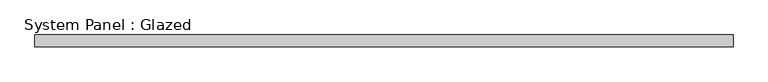
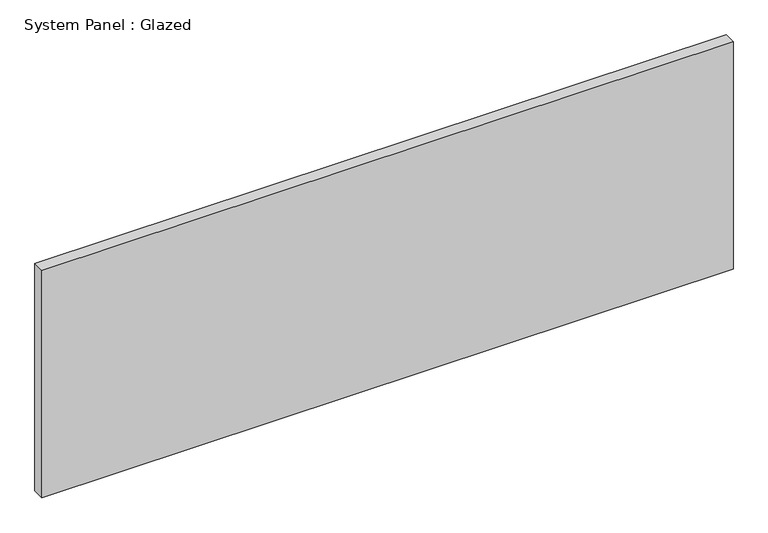
"""IFC4 building model written with IfcOpenShell, lengths in millimetres: plate geometry, System Panel : Glazed."""

from ifc_helpers import new_model, si_unit, origin, origin_with_axes, place, context, project, spatial, polyline, outline, extrude, source, transform, mapped, element, save


def system_panel_glazed_f9c14314(model_context):
    return source(origin(), model_context, "Body", "SweptSolid", [
        extrude(outline(polyline([(739.3657433, -44.45), (-739.3657433, -44.45), (-739.3657433, -19.05), (739.3657433, -19.05), (739.3657433, -44.45)])), origin_with_axes(), (0.0, 0.0, 1.0), 514.35),
    ])


if __name__ == "__main__":
    model = new_model("IFC4")
    model_context = context("Model", 3, world=origin())
    ifc_project = project(units=[si_unit("LENGTHUNIT", "METRE", prefix="MILLI")], contexts=[model_context])
    site = spatial("IfcSite", under=ifc_project)
    building = spatial("IfcBuilding", under=site)
    placement = place(None, origin())
    system_panel_glazed_shape = system_panel_glazed_f9c14314(model_context)
    element("IfcPlate", 1, ObjectType="System Panel : Glazed", at=placement, inside=building, context=model_context, shape_type="MappedRepresentation", body=[
        mapped(system_panel_glazed_shape, transform((0.0, 0.0, 0.0), x_axis=(1.0, 0.0, 0.0), y_axis=(0.0, 1.0, 0.0), z_axis=(0.0, 0.0, 1.0))),
    ])
    save(model, "model.ifc")

# Revit data of these elements
# Type "System Panel : Glazed"
#   Construction Type Id = "GSP4R"
#   Analytic Construction = "1/8 in Pilkington single glazing"
#   Visual Light Transmittance = 0.9
#   Solar Heat Gain Coefficient = 0.86
#   Heat Transfer Coefficient (U) = 1.18115 BTU/(h·ft²·°F)
# Element 1 (IfcPlate, "System Panel : Glazed")
#   Materials on its faces: "Glass"
# Materials
#   "Glass": class "Glass", colour RGB 0 128 192, transparency 0.75, Description = "Soda Lime Glass", Cost = 0
